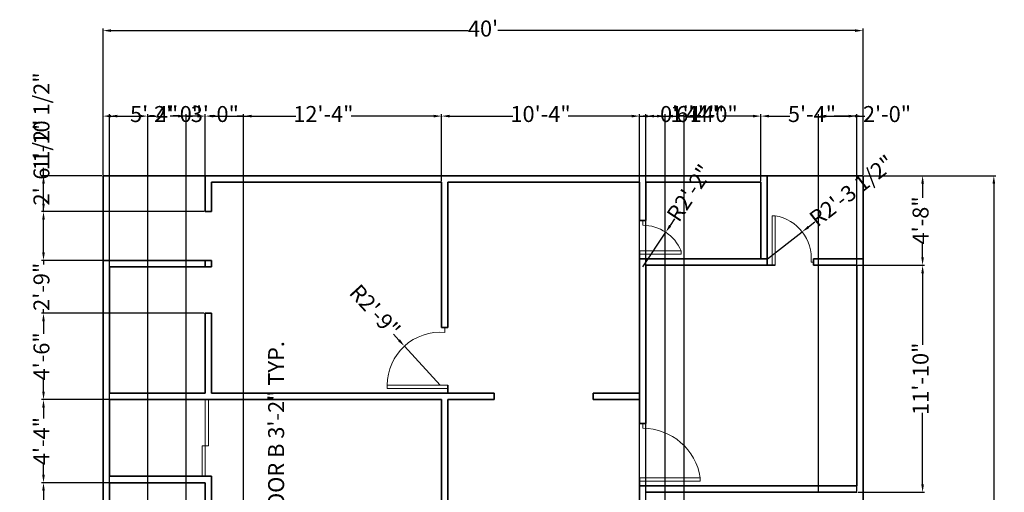
# Model space of a CAD drawing. Units: inches. Extents: x 2565 to 3182, y 2168 to 2957.
# Tile 3 of 3: x 2565 to 3182, y 2662 to 2957. Entities that reach past the tile are written whole.
import ezdxf

# ---------------------------------------------------------------- set-up
doc = ezdxf.new("R2010")
doc.units = ezdxf.units.IN
for name, color, linetype, lineweight in [('A-ANNO-DIMS', 2, 'Continuous', 13), ('A-DOOR', 4, 'Continuous', 18), ('A-GLAZ', 3, 'Continuous', 18), ('A-WALL', 7, 'Continuous', 35)]:
    doc.layers.add(name, color=color, linetype=linetype, lineweight=lineweight)
doc.styles.get("Standard").update_dxf_attribs({"font": 'arial.ttf'})
doc.dimstyles.new('ISO-25', dxfattribs={"dimtxt": 10, "dimasz": 5, "dimexe": 1.25, "dimexo": 0.625, "dimtad": 0, "dimdec": 0, "dimrnd": 10, "dimlunit": 3, "dimtxsty": 'Standard', "dimcen": 2.5, "dimadec": 0, "dimazin": 0, "dimtfac": 1, "dimtdec": 0, "dimtmove": 0, "dimatfit": 3, "dimfxl": 1, "dimarcsym": 0})

# ---------------------------------------------------------------- blocks, each defined once
blk = doc.blocks.new('*D2')
at = {"layer": 'A-ANNO-DIMS', "color": 0, "lineweight": -2, "transparency": 16777216}
for p, q in [((3094.05, 2859.77), (3176.57, 2859.77)), ((3175.32, 2854.77), (3175.32, 2553.57)), ((3175.32, 2216.77), (3175.32, 2517.97)), ((3094.05, 2211.77), (3176.57, 2211.77))]:
    blk.add_line(p, q, dxfattribs=at)
at = {"layer": 'A-ANNO-DIMS', "color": 0, "transparency": 16777216}
for points in [[(3174.49, 2854.77), (3176.15, 2854.77), (3175.32, 2859.77)], [(3174.49, 2216.77), (3176.15, 2216.77), (3175.32, 2211.77)]]:
    blk.add_solid(points, dxfattribs=at)
at = {"layer": 'Defpoints', "color": 0, "transparency": 16777216}
for p in [(3093.43, 2859.77), (3093.43, 2211.77), (3175.32, 2211.77)]:
    blk.add_point(p, dxfattribs=at)
at = {"layer": 'A-ANNO-DIMS', "color": 0, "transparency": 16777216, "insert": (3175.32, 2535.77), "char_height": 10, "attachment_point": 5, "rotation": 90}
blk.add_mtext('54\'-2"', dxfattribs=at)
blk = doc.blocks.new('*D3')
at = {"layer": 'A-ANNO-DIMS', "color": 0, "lineweight": -2, "transparency": 16777216}
for p, q in [((2617.43, 2860.39), (2617.43, 2951.77)), ((2622.43, 2950.52), (2846.12, 2950.52)), ((3088.43, 2950.52), (2864.74, 2950.52)), ((3093.43, 2860.39), (3093.43, 2951.77))]:
    blk.add_line(p, q, dxfattribs=at)
at = {"layer": 'A-ANNO-DIMS', "color": 0, "transparency": 16777216}
for points in [[(2622.43, 2951.35), (2622.43, 2949.69), (2617.43, 2950.52)], [(3088.43, 2951.35), (3088.43, 2949.69), (3093.43, 2950.52)]]:
    blk.add_solid(points, dxfattribs=at)
at = {"layer": 'Defpoints', "color": 0, "transparency": 16777216}
for p in [(3093.43, 2950.52), (2617.43, 2859.77), (3093.43, 2859.77)]:
    blk.add_point(p, dxfattribs=at)
at = {"layer": 'A-ANNO-DIMS', "color": 0, "transparency": 16777216, "insert": (2855.43, 2950.52), "char_height": 10, "attachment_point": 5}
blk.add_mtext("40'", dxfattribs=at)
blk = doc.blocks.new('DOOR-SWING-36-OPENING-39')
for p, q in [((2, 36), (2, 33)), ((38, 2), (0, 2)), ((0, 2), (0, 0)), ((2, 0), (38, 0)), ((38, 0), (38, 2))]:
    blk.add_line(p, q)
blk.add_arc((2, -3.4), 36.4, 8.53579, 90)
blk = doc.blocks.new('*D9')
at = {"layer": 'A-ANNO-DIMS', "color": 0, "lineweight": -2, "transparency": 16777216}
for p, q in [((2722.05, 2633.77), (2728.38, 2633.77)), ((2727.13, 2633.77), (2727.13, 2638.77)), ((2727.13, 2600.77), (2727.13, 2628.77)), ((2722.05, 2595.77), (2728.38, 2595.77))]:
    blk.add_line(p, q, dxfattribs=at)
at = {"layer": 'A-ANNO-DIMS', "color": 0, "transparency": 16777216}
for points in [[(2726.3, 2628.77), (2727.96, 2628.77), (2727.13, 2633.77)], [(2726.3, 2600.77), (2727.96, 2600.77), (2727.13, 2595.77)]]:
    blk.add_solid(points, dxfattribs=at)
at = {"layer": 'Defpoints', "color": 0, "transparency": 16777216}
for p in [(2721.43, 2633.77), (2727.13, 2633.77), (2721.43, 2595.77)]:
    blk.add_point(p, dxfattribs=at)
at = {"layer": 'A-ANNO-DIMS', "color": 0, "transparency": 16777216, "insert": (2727.13, 2699.12), "char_height": 10, "attachment_point": 5, "rotation": 90}
blk.add_mtext('DOOR B 3\'-2" TYP.', dxfattribs=at)
blk = doc.blocks.new('*D13')
at = {"layer": 'A-ANNO-DIMS', "color": 0, "lineweight": -2, "transparency": 16777216}
for p, q in [((2617.43, 2860.39), (2617.43, 2898.3)), ((2681.43, 2860.39), (2681.43, 2898.3)), ((2622.43, 2897.05), (2635.51, 2897.05)), ((2676.43, 2897.05), (2663.35, 2897.05))]:
    blk.add_line(p, q, dxfattribs=at)
at = {"layer": 'A-ANNO-DIMS', "color": 0, "transparency": 16777216}
for points in [[(2622.43, 2897.88), (2622.43, 2896.21), (2617.43, 2897.05)], [(2676.43, 2897.88), (2676.43, 2896.21), (2681.43, 2897.05)]]:
    blk.add_solid(points, dxfattribs=at)
at = {"layer": 'Defpoints', "color": 0, "transparency": 16777216}
for p in [(2681.43, 2897.05), (2617.43, 2859.77), (2681.43, 2859.77)]:
    blk.add_point(p, dxfattribs=at)
at = {"layer": 'A-ANNO-DIMS', "color": 0, "transparency": 16777216, "insert": (2649.43, 2897.05), "char_height": 10, "attachment_point": 5}
blk.add_mtext('5\'-4"', dxfattribs=at)
blk = doc.blocks.new('*D14')
at = {"layer": 'A-ANNO-DIMS', "color": 0, "lineweight": -2, "transparency": 16777216}
for p, q in [((2681.43, 2860.39), (2681.43, 2898.3)), ((2829.43, 2856.39), (2829.43, 2898.3)), ((2686.43, 2897.05), (2738.1, 2897.05)), ((2824.43, 2897.05), (2772.76, 2897.05))]:
    blk.add_line(p, q, dxfattribs=at)
at = {"layer": 'A-ANNO-DIMS', "color": 0, "transparency": 16777216}
for points in [[(2686.43, 2897.88), (2686.43, 2896.21), (2681.43, 2897.05)], [(2824.43, 2897.88), (2824.43, 2896.21), (2829.43, 2897.05)]]:
    blk.add_solid(points, dxfattribs=at)
at = {"layer": 'Defpoints', "color": 0, "transparency": 16777216}
for p in [(2829.43, 2897.05), (2681.43, 2859.77), (2829.43, 2855.77)]:
    blk.add_point(p, dxfattribs=at)
at = {"layer": 'A-ANNO-DIMS', "color": 0, "transparency": 16777216, "insert": (2755.43, 2897.05), "char_height": 10, "attachment_point": 5}
blk.add_mtext('12\'-4"', dxfattribs=at)
blk = doc.blocks.new('*D15')
at = {"layer": 'A-ANNO-DIMS', "color": 0, "lineweight": -2, "transparency": 16777216}
for p, q in [((2829.43, 2856.39), (2829.43, 2898.3)), ((2953.43, 2856.39), (2953.43, 2898.3)), ((2834.43, 2897.05), (2874.1, 2897.05)), ((2948.43, 2897.05), (2908.76, 2897.05))]:
    blk.add_line(p, q, dxfattribs=at)
at = {"layer": 'A-ANNO-DIMS', "color": 0, "transparency": 16777216}
for points in [[(2834.43, 2897.88), (2834.43, 2896.21), (2829.43, 2897.05)], [(2948.43, 2897.88), (2948.43, 2896.21), (2953.43, 2897.05)]]:
    blk.add_solid(points, dxfattribs=at)
at = {"layer": 'Defpoints', "color": 0, "transparency": 16777216}
for p in [(2953.43, 2897.05), (2829.43, 2855.77), (2953.43, 2855.77)]:
    blk.add_point(p, dxfattribs=at)
at = {"layer": 'A-ANNO-DIMS', "color": 0, "transparency": 16777216, "insert": (2891.43, 2897.05), "char_height": 10, "attachment_point": 5}
blk.add_mtext('10\'-4"', dxfattribs=at)
blk = doc.blocks.new('*D16')
at = {"layer": 'A-ANNO-DIMS', "color": 0, "lineweight": -2, "transparency": 16777216}
for p, q in [((2953.43, 2856.39), (2953.43, 2898.3)), ((3029.43, 2856.39), (3029.43, 2898.3)), ((2958.43, 2897.05), (2977.49, 2897.05)), ((3024.43, 2897.05), (3005.37, 2897.05))]:
    blk.add_line(p, q, dxfattribs=at)
at = {"layer": 'A-ANNO-DIMS', "color": 0, "transparency": 16777216}
for points in [[(2958.43, 2897.88), (2958.43, 2896.21), (2953.43, 2897.05)], [(3024.43, 2897.88), (3024.43, 2896.21), (3029.43, 2897.05)]]:
    blk.add_solid(points, dxfattribs=at)
at = {"layer": 'Defpoints', "color": 0, "transparency": 16777216}
for p in [(3029.43, 2897.05), (2953.43, 2855.77), (3029.43, 2855.77)]:
    blk.add_point(p, dxfattribs=at)
at = {"layer": 'A-ANNO-DIMS', "color": 0, "transparency": 16777216, "insert": (2991.43, 2897.05), "char_height": 10, "attachment_point": 5}
blk.add_mtext('6\'-4"', dxfattribs=at)
blk = doc.blocks.new('*D17')
at = {"layer": 'A-ANNO-DIMS', "color": 0, "lineweight": -2, "transparency": 16777216}
for p, q in [((3029.43, 2856.39), (3029.43, 2898.3)), ((3093.43, 2860.39), (3093.43, 2898.3)), ((3034.43, 2897.05), (3047.51, 2897.05)), ((3088.43, 2897.05), (3075.35, 2897.05))]:
    blk.add_line(p, q, dxfattribs=at)
at = {"layer": 'A-ANNO-DIMS', "color": 0, "transparency": 16777216}
for points in [[(3034.43, 2897.88), (3034.43, 2896.21), (3029.43, 2897.05)], [(3088.43, 2897.88), (3088.43, 2896.21), (3093.43, 2897.05)]]:
    blk.add_solid(points, dxfattribs=at)
at = {"layer": 'Defpoints', "color": 0, "transparency": 16777216}
for p in [(3093.43, 2897.05), (3029.43, 2855.77), (3093.43, 2859.77)]:
    blk.add_point(p, dxfattribs=at)
at = {"layer": 'A-ANNO-DIMS', "color": 0, "transparency": 16777216, "insert": (3061.43, 2897.05), "char_height": 10, "attachment_point": 5}
blk.add_mtext('5\'-4"', dxfattribs=at)
blk = doc.blocks.new('*D23')
at = {"layer": 'A-ANNO-DIMS', "color": 0, "lineweight": -2, "transparency": 16777216}
for p, q in [((2620.8, 2667.77), (2578.9, 2667.77)), ((2580.15, 2662.77), (2580.15, 2645.71)), ((2580.15, 2600.77), (2580.15, 2617.82)), ((2620.8, 2595.77), (2578.9, 2595.77))]:
    blk.add_line(p, q, dxfattribs=at)
at = {"layer": 'A-ANNO-DIMS', "color": 0, "transparency": 16777216}
for points in [[(2579.32, 2662.77), (2580.98, 2662.77), (2580.15, 2667.77)], [(2579.32, 2600.77), (2580.98, 2600.77), (2580.15, 2595.77)]]:
    blk.add_solid(points, dxfattribs=at)
at = {"layer": 'Defpoints', "color": 0, "transparency": 16777216}
for p in [(2580.15, 2667.77), (2621.43, 2667.77), (2621.43, 2595.77)]:
    blk.add_point(p, dxfattribs=at)
at = {"layer": 'A-ANNO-DIMS', "color": 0, "transparency": 16777216, "insert": (2580.15, 2631.77), "char_height": 10, "attachment_point": 5, "rotation": 90}
blk.add_mtext('6\'-0"', dxfattribs=at)
blk = doc.blocks.new('*D24')
at = {"layer": 'A-ANNO-DIMS', "color": 0, "lineweight": -2, "transparency": 16777216}
for p, q in [((2620.8, 2719.77), (2578.9, 2719.77)), ((2580.15, 2714.77), (2580.15, 2707.89)), ((2580.15, 2672.77), (2580.15, 2679.65)), ((2620.8, 2667.77), (2578.9, 2667.77))]:
    blk.add_line(p, q, dxfattribs=at)
at = {"layer": 'A-ANNO-DIMS', "color": 0, "transparency": 16777216}
for points in [[(2579.32, 2714.77), (2580.98, 2714.77), (2580.15, 2719.77)], [(2579.32, 2672.77), (2580.98, 2672.77), (2580.15, 2667.77)]]:
    blk.add_solid(points, dxfattribs=at)
at = {"layer": 'Defpoints', "color": 0, "transparency": 16777216}
for p in [(2580.15, 2719.77), (2621.43, 2719.77), (2621.43, 2667.77)]:
    blk.add_point(p, dxfattribs=at)
at = {"layer": 'A-ANNO-DIMS', "color": 0, "transparency": 16777216, "insert": (2580.15, 2693.77), "char_height": 10, "attachment_point": 5, "rotation": 90}
blk.add_mtext('4\'-4"', dxfattribs=at)
blk = doc.blocks.new('*D25')
at = {"layer": 'A-ANNO-DIMS', "color": 0, "lineweight": -2, "transparency": 16777216}
for p, q in [((2680.8, 2773.77), (2578.9, 2773.77)), ((2580.15, 2768.77), (2580.15, 2760.89)), ((2580.15, 2724.77), (2580.15, 2732.65)), ((2620.8, 2719.77), (2578.9, 2719.77))]:
    blk.add_line(p, q, dxfattribs=at)
at = {"layer": 'A-ANNO-DIMS', "color": 0, "transparency": 16777216}
for points in [[(2579.32, 2768.77), (2580.98, 2768.77), (2580.15, 2773.77)], [(2579.32, 2724.77), (2580.98, 2724.77), (2580.15, 2719.77)]]:
    blk.add_solid(points, dxfattribs=at)
at = {"layer": 'Defpoints', "color": 0, "transparency": 16777216}
for p in [(2580.15, 2773.77), (2681.43, 2773.77), (2621.43, 2719.77)]:
    blk.add_point(p, dxfattribs=at)
at = {"layer": 'A-ANNO-DIMS', "color": 0, "transparency": 16777216, "insert": (2580.15, 2746.77), "char_height": 10, "attachment_point": 5, "rotation": 90}
blk.add_mtext('4\'-6"', dxfattribs=at)
blk = doc.blocks.new('*D26')
at = {"layer": 'A-ANNO-DIMS', "color": 0, "lineweight": -2, "transparency": 16777216}
for p, q in [((2580.15, 2811.77), (2580.15, 2816.77)), ((2616.8, 2806.77), (2578.9, 2806.77)), ((2580.15, 2806.77), (2580.15, 2804.27)), ((2580.15, 2773.77), (2580.15, 2776.27)), ((2680.8, 2773.77), (2578.9, 2773.77)), ((2580.15, 2768.77), (2580.15, 2763.77))]:
    blk.add_line(p, q, dxfattribs=at)
at = {"layer": 'A-ANNO-DIMS', "color": 0, "transparency": 16777216}
for points in [[(2579.32, 2811.77), (2580.98, 2811.77), (2580.15, 2806.77)], [(2579.32, 2768.77), (2580.98, 2768.77), (2580.15, 2773.77)]]:
    blk.add_solid(points, dxfattribs=at)
at = {"layer": 'Defpoints', "color": 0, "transparency": 16777216}
for p in [(2580.15, 2806.77), (2617.43, 2806.77), (2681.43, 2773.77)]:
    blk.add_point(p, dxfattribs=at)
at = {"layer": 'A-ANNO-DIMS', "color": 0, "transparency": 16777216, "insert": (2580.15, 2790.27), "char_height": 10, "attachment_point": 5, "rotation": 90}
blk.add_mtext('2\'-9"', dxfattribs=at)
blk = doc.blocks.new('*D27')
at = {"layer": 'A-ANNO-DIMS', "color": 0, "lineweight": -2, "transparency": 16777216}
for p, q in [((2680.8, 2837.35), (2578.9, 2837.35)), ((2580.15, 2837.35), (2580.15, 2842.35)), ((2580.15, 2811.77), (2580.15, 2832.35)), ((2616.8, 2806.77), (2578.9, 2806.77))]:
    blk.add_line(p, q, dxfattribs=at)
at = {"layer": 'A-ANNO-DIMS', "color": 0, "transparency": 16777216}
for points in [[(2579.32, 2832.35), (2580.98, 2832.35), (2580.15, 2837.35)], [(2579.32, 2811.77), (2580.98, 2811.77), (2580.15, 2806.77)]]:
    blk.add_solid(points, dxfattribs=at)
at = {"layer": 'Defpoints', "color": 0, "transparency": 16777216}
for p in [(2580.15, 2837.35), (2681.43, 2837.35), (2617.43, 2806.77)]:
    blk.add_point(p, dxfattribs=at)
at = {"layer": 'A-ANNO-DIMS', "color": 0, "transparency": 16777216, "insert": (2580.15, 2868), "char_height": 10, "attachment_point": 5, "rotation": 90}
blk.add_mtext('2\'-6 1/2"', dxfattribs=at)
blk = doc.blocks.new('*D28')
at = {"layer": 'A-ANNO-DIMS', "color": 0, "lineweight": -2, "transparency": 16777216}
for p, q in [((2580.15, 2859.77), (2580.15, 2864.77)), ((2616.8, 2859.77), (2578.9, 2859.77)), ((2580.15, 2842.35), (2580.15, 2854.77)), ((2680.8, 2837.35), (2578.9, 2837.35))]:
    blk.add_line(p, q, dxfattribs=at)
at = {"layer": 'A-ANNO-DIMS', "color": 0, "transparency": 16777216}
for points in [[(2579.32, 2854.77), (2580.98, 2854.77), (2580.15, 2859.77)], [(2579.32, 2842.35), (2580.98, 2842.35), (2580.15, 2837.35)]]:
    blk.add_solid(points, dxfattribs=at)
at = {"layer": 'Defpoints', "color": 0, "transparency": 16777216}
for p in [(2580.15, 2859.77), (2617.43, 2859.77), (2681.43, 2837.35)]:
    blk.add_point(p, dxfattribs=at)
at = {"layer": 'A-ANNO-DIMS', "color": 0, "transparency": 16777216, "insert": (2580.15, 2893.75), "char_height": 10, "attachment_point": 5, "rotation": 90}
blk.add_mtext('1\'-10 1/2"', dxfattribs=at)
blk = doc.blocks.new('*D34')
at = {"layer": 'A-ANNO-DIMS', "color": 0, "lineweight": -2, "transparency": 16777216}
for p, q in [((3090.05, 2803.77), (3131.96, 2803.77)), ((3130.71, 2798.77), (3130.71, 2753.98)), ((3130.71, 2666.77), (3130.71, 2711.55)), ((3090.05, 2661.77), (3131.96, 2661.77))]:
    blk.add_line(p, q, dxfattribs=at)
at = {"layer": 'A-ANNO-DIMS', "color": 0, "transparency": 16777216}
for points in [[(3129.88, 2798.77), (3131.54, 2798.77), (3130.71, 2803.77)], [(3129.88, 2666.77), (3131.54, 2666.77), (3130.71, 2661.77)]]:
    blk.add_solid(points, dxfattribs=at)
at = {"layer": 'Defpoints', "color": 0, "transparency": 16777216}
for p in [(3089.43, 2803.77), (3130.71, 2803.77), (3089.43, 2661.77)]:
    blk.add_point(p, dxfattribs=at)
at = {"layer": 'A-ANNO-DIMS', "color": 0, "transparency": 16777216, "insert": (3130.71, 2732.77), "char_height": 10, "attachment_point": 5, "rotation": 90}
blk.add_mtext('11\'-10"', dxfattribs=at)
blk = doc.blocks.new('*D35')
at = {"layer": 'A-ANNO-DIMS', "color": 0, "lineweight": -2, "transparency": 16777216}
for p, q in [((3094.05, 2859.77), (3131.96, 2859.77)), ((3130.71, 2854.77), (3130.71, 2845.89)), ((3130.71, 2808.77), (3130.71, 2817.65)), ((3090.05, 2803.77), (3131.96, 2803.77))]:
    blk.add_line(p, q, dxfattribs=at)
at = {"layer": 'A-ANNO-DIMS', "color": 0, "transparency": 16777216}
for points in [[(3129.88, 2854.77), (3131.54, 2854.77), (3130.71, 2859.77)], [(3129.88, 2808.77), (3131.54, 2808.77), (3130.71, 2803.77)]]:
    blk.add_solid(points, dxfattribs=at)
at = {"layer": 'Defpoints', "color": 0, "transparency": 16777216}
for p in [(3093.43, 2859.77), (3130.71, 2859.77), (3089.43, 2803.77)]:
    blk.add_point(p, dxfattribs=at)
at = {"layer": 'A-ANNO-DIMS', "color": 0, "transparency": 16777216, "insert": (3130.71, 2831.77), "char_height": 10, "attachment_point": 5, "rotation": 90}
blk.add_mtext('4\'-8"', dxfattribs=at)
blk = doc.blocks.new('*D42')
at = {"layer": 'A-ANNO-DIMS', "color": 0, "lineweight": -2, "transparency": 16777216}
for p, q in [((2669.43, 2552.39), (2669.43, 2898.3)), ((2705.43, 2552.39), (2705.43, 2898.3)), ((2664.43, 2897.05), (2659.43, 2897.05)), ((2669.43, 2897.05), (2673.52, 2897.05)), ((2705.43, 2897.05), (2701.34, 2897.05)), ((2710.43, 2897.05), (2715.43, 2897.05))]:
    blk.add_line(p, q, dxfattribs=at)
at = {"layer": 'A-ANNO-DIMS', "color": 0, "transparency": 16777216}
for points in [[(2664.43, 2897.88), (2664.43, 2896.21), (2669.43, 2897.05)], [(2710.43, 2897.88), (2710.43, 2896.21), (2705.43, 2897.05)]]:
    blk.add_solid(points, dxfattribs=at)
at = {"layer": 'Defpoints', "color": 0, "transparency": 16777216}
for p in [(2705.43, 2897.05), (2669.43, 2551.77), (2705.43, 2551.77)]:
    blk.add_point(p, dxfattribs=at)
at = {"layer": 'A-ANNO-DIMS', "color": 0, "transparency": 16777216, "insert": (2687.43, 2897.05), "char_height": 10, "attachment_point": 5}
blk.add_mtext('3\'-0"', dxfattribs=at)
blk = doc.blocks.new('*D43')
at = {"layer": 'A-ANNO-DIMS', "color": 0, "lineweight": -2, "transparency": 16777216}
for p, q in [((2621.43, 2548.39), (2621.43, 2898.3)), ((2645.43, 2548.39), (2645.43, 2898.3)), ((2626.43, 2897.05), (2640.43, 2897.05)), ((2645.43, 2897.05), (2650.43, 2897.05))]:
    blk.add_line(p, q, dxfattribs=at)
at = {"layer": 'A-ANNO-DIMS', "color": 0, "transparency": 16777216}
for points in [[(2626.43, 2897.88), (2626.43, 2896.21), (2621.43, 2897.05)], [(2640.43, 2897.88), (2640.43, 2896.21), (2645.43, 2897.05)]]:
    blk.add_solid(points, dxfattribs=at)
at = {"layer": 'Defpoints', "color": 0, "transparency": 16777216}
for p in [(2645.43, 2897.05), (2621.43, 2547.77), (2645.43, 2547.77)]:
    blk.add_point(p, dxfattribs=at)
at = {"layer": 'A-ANNO-DIMS', "color": 0, "transparency": 16777216, "insert": (2664.43, 2897.05), "char_height": 10, "attachment_point": 5}
blk.add_mtext('2\'-0"', dxfattribs=at)
blk = doc.blocks.new('*D52')
at = {"layer": 'A-ANNO-DIMS', "color": 0, "lineweight": -2, "transparency": 16777216}
for p, q in [((2953.43, 2586.39), (2953.43, 2898.3)), ((2969.43, 2586.39), (2969.43, 2898.3)), ((2958.43, 2897.05), (2964.43, 2897.05)), ((2969.43, 2897.05), (2974.43, 2897.05))]:
    blk.add_line(p, q, dxfattribs=at)
at = {"layer": 'A-ANNO-DIMS', "color": 0, "transparency": 16777216}
for points in [[(2958.43, 2897.88), (2958.43, 2896.21), (2953.43, 2897.05)], [(2964.43, 2897.88), (2964.43, 2896.21), (2969.43, 2897.05)]]:
    blk.add_solid(points, dxfattribs=at)
at = {"layer": 'Defpoints', "color": 0, "transparency": 16777216}
for p in [(2969.43, 2897.05), (2953.43, 2585.77), (2969.43, 2585.77)]:
    blk.add_point(p, dxfattribs=at)
at = {"layer": 'A-ANNO-DIMS', "color": 0, "transparency": 16777216, "insert": (2987.87, 2897.05), "char_height": 10, "attachment_point": 5}
blk.add_mtext('1\'-4"', dxfattribs=at)
blk = doc.blocks.new('*D53')
at = {"layer": 'A-ANNO-DIMS', "color": 0, "lineweight": -2, "transparency": 16777216}
for p, q in [((2969.43, 2586.39), (2969.43, 2898.3)), ((2981.43, 2586.39), (2981.43, 2898.3)), ((2974.43, 2897.05), (2976.43, 2897.05)), ((2981.43, 2897.05), (2986.43, 2897.05))]:
    blk.add_line(p, q, dxfattribs=at)
at = {"layer": 'A-ANNO-DIMS', "color": 0, "transparency": 16777216}
for points in [[(2974.43, 2897.88), (2974.43, 2896.21), (2969.43, 2897.05)], [(2976.43, 2897.88), (2976.43, 2896.21), (2981.43, 2897.05)]]:
    blk.add_solid(points, dxfattribs=at)
at = {"layer": 'Defpoints', "color": 0, "transparency": 16777216}
for p in [(2981.43, 2897.05), (2969.43, 2585.77), (2981.43, 2585.77)]:
    blk.add_point(p, dxfattribs=at)
at = {"layer": 'A-ANNO-DIMS', "color": 0, "transparency": 16777216, "insert": (2999.87, 2897.05), "char_height": 10, "attachment_point": 5}
blk.add_mtext('1\'-0"', dxfattribs=at)
blk = doc.blocks.new('*D57')
at = {"layer": 'A-ANNO-DIMS', "color": 0, "lineweight": -2, "transparency": 16777216}
for p, q in [((3065.43, 2662.39), (3065.43, 2898.3)), ((3089.43, 2662.39), (3089.43, 2898.3)), ((3070.43, 2897.05), (3084.43, 2897.05)), ((3089.43, 2897.05), (3094.43, 2897.05))]:
    blk.add_line(p, q, dxfattribs=at)
at = {"layer": 'A-ANNO-DIMS', "color": 0, "transparency": 16777216}
for points in [[(3070.43, 2897.88), (3070.43, 2896.21), (3065.43, 2897.05)], [(3084.43, 2897.88), (3084.43, 2896.21), (3089.43, 2897.05)]]:
    blk.add_solid(points, dxfattribs=at)
at = {"layer": 'Defpoints', "color": 0, "transparency": 16777216}
for p in [(3089.43, 2897.05), (3065.43, 2661.77), (3089.43, 2661.77)]:
    blk.add_point(p, dxfattribs=at)
at = {"layer": 'A-ANNO-DIMS', "color": 0, "transparency": 16777216, "insert": (3108.43, 2897.05), "char_height": 10, "attachment_point": 5}
blk.add_mtext('2\'-0"', dxfattribs=at)
blk = doc.blocks.new('*D59')
at = {"layer": 'A-ANNO-DIMS', "color": 0, "lineweight": -2, "transparency": 16777216}
for p, q in [((2953.43, 2623.39), (2953.43, 2898.3)), ((2957.43, 2623.39), (2957.43, 2898.3)), ((2948.43, 2897.05), (2943.43, 2897.05)), ((2953.43, 2897.05), (2957.43, 2897.05)), ((2962.43, 2897.05), (2967.43, 2897.05))]:
    blk.add_line(p, q, dxfattribs=at)
at = {"layer": 'A-ANNO-DIMS', "color": 0, "transparency": 16777216}
for points in [[(2948.43, 2897.88), (2948.43, 2896.21), (2953.43, 2897.05)], [(2962.43, 2897.88), (2962.43, 2896.21), (2957.43, 2897.05)]]:
    blk.add_solid(points, dxfattribs=at)
at = {"layer": 'Defpoints', "color": 0, "transparency": 16777216}
for p in [(2957.43, 2897.05), (2953.43, 2622.77), (2957.43, 2622.77)]:
    blk.add_point(p, dxfattribs=at)
at = {"layer": 'A-ANNO-DIMS', "color": 0, "transparency": 16777216, "insert": (2981.35, 2897.05), "char_height": 10, "attachment_point": 5}
blk.add_mtext('0\'-4"', dxfattribs=at)
blk = doc.blocks.new('*D65')
at = {"layer": 'A-ANNO-DIMS', "color": 0, "lineweight": -2, "transparency": 16777216}
for p, q in [((2799.41, 2760.56), (2802.79, 2756.87)), ((2828.55, 2728.77), (2806.17, 2753.19))]:
    blk.add_line(p, q, dxfattribs=at)
at = {"layer": 'A-ANNO-DIMS', "color": 0, "transparency": 16777216}
blk.add_solid([(2803.41, 2757.44), (2802.18, 2756.31), (2806.17, 2753.19)], dxfattribs=at)
at = {"layer": 'Defpoints', "color": 0, "transparency": 16777216}
for p in [(2806.17, 2753.19), (2828.55, 2728.77)]:
    blk.add_point(p, dxfattribs=at)
at = {"layer": 'A-ANNO-DIMS', "color": 0, "transparency": 16777216, "insert": (2786.78, 2774.34), "char_height": 10, "attachment_point": 5, "rotation": 312.51029}
blk.add_mtext('R2\'-9"', dxfattribs=at)
blk = doc.blocks.new('*D69')
at = {"layer": 'A-ANNO-DIMS', "color": 0, "lineweight": -2, "transparency": 16777216}
for p, q in [((3063.17, 2830.74), (3059.22, 2827.67)), ((3033.67, 2807.85), (3055.27, 2824.61))]:
    blk.add_line(p, q, dxfattribs=at)
at = {"layer": 'A-ANNO-DIMS', "color": 0, "transparency": 16777216}
blk.add_solid([(3058.71, 2828.33), (3059.73, 2827.01), (3055.27, 2824.61)], dxfattribs=at)
at = {"layer": 'Defpoints', "color": 0, "transparency": 16777216}
for p in [(3055.27, 2824.61), (3033.67, 2807.85)]:
    blk.add_point(p, dxfattribs=at)
at = {"layer": 'A-ANNO-DIMS', "color": 0, "transparency": 16777216, "insert": (3087.15, 2849.34), "char_height": 10, "attachment_point": 5, "rotation": 37.80584}
blk.add_mtext('R2\'-3 1/2"', dxfattribs=at)
blk = doc.blocks.new('*D71')
at = {"layer": 'A-ANNO-DIMS', "color": 0, "lineweight": -2, "transparency": 16777216}
for p, q in [((2975.4, 2832.72), (2972.62, 2828.56)), ((2955.43, 2802.77), (2969.85, 2824.4))]:
    blk.add_line(p, q, dxfattribs=at)
at = {"layer": 'A-ANNO-DIMS', "color": 0, "transparency": 16777216}
blk.add_solid([(2971.93, 2829.02), (2973.32, 2828.1), (2969.85, 2824.4)], dxfattribs=at)
at = {"layer": 'Defpoints', "color": 0, "transparency": 16777216}
for p in [(2969.85, 2824.4), (2955.43, 2802.77)]:
    blk.add_point(p, dxfattribs=at)
at = {"layer": 'A-ANNO-DIMS', "color": 0, "transparency": 16777216, "insert": (2985.77, 2848.28), "char_height": 10, "attachment_point": 5, "rotation": 56.31031}
blk.add_mtext('R2\'-2"', dxfattribs=at)

msp = doc.modelspace()

# ---------------------------------------------------------------- linework, layer by layer
at = {"layer": 'A-DOOR'}
for p, q in [((2955.43, 2831.77), (2955.43, 2828.77)), ((3036.43, 2805.77), (3036.43, 2834.77)), ((3036.43, 2834.77), (3038.43, 2834.77)), ((3038.43, 2834.77), (3038.43, 2803.77)), ((2979.43, 2812.77), (2953.43, 2812.77)), ((2953.43, 2812.77), (2953.43, 2810.77)), ((2979.43, 2810.77), (2979.43, 2812.77)), ((2953.43, 2810.77), (2957.43, 2810.77)), ((2955.43, 2810.77), (2979.43, 2810.77)), ((3036.43, 2803.77), (3036.43, 2807.77)), ((3062.43, 2805.77), (3060.93, 2805.77)), ((3038.43, 2803.77), (3036.43, 2803.77)), ((2831.43, 2764.77), (2831.43, 2761.77)), ((2795.43, 2726.77), (2795.43, 2728.77)), ((2795.43, 2728.77), (2833.43, 2728.77)), ((2831.43, 2726.77), (2795.43, 2726.77)), ((2833.43, 2726.77), (2826.72, 2726.77)), ((2829.43, 2728.77), (2833.43, 2728.77)), ((2833.43, 2728.77), (2833.43, 2726.77)), ((2953.43, 2668.77), (2957.43, 2668.77))]:
    msp.add_line(p, q, dxfattribs=at)
for centre, radius, start, end in [((3033.67, 2807.85), 27.33, 355.631, 79.98206), ((2955.43, 2802.77), 26, 22.61986, 90), ((2828.55, 2728.77), 33.12, 85.02089, 180)]:
    msp.add_arc(centre, radius, start, end, dxfattribs=at)
at = {"layer": 'A-GLAZ'}
for p, q in [((2681.43, 2719.77), (2681.43, 2690.77)), ((2683.43, 2719.77), (2681.43, 2719.77)), ((2683.43, 2690.77), (2683.43, 2719.77)), ((2681.43, 2690.77), (2679.43, 2690.77)), ((2679.43, 2690.77), (2679.43, 2671.77)), ((2681.43, 2690.77), (2683.43, 2690.77)), ((2681.43, 2671.78), (2681.43, 2690.77)), ((2679.43, 2671.77), (2681.43, 2671.78))]:
    msp.add_line(p, q, dxfattribs=at)
at = {"layer": 'A-WALL'}
for p, q in [((3093.43, 2859.77), (2617.43, 2859.77)), ((2617.43, 2859.77), (2617.43, 2211.77)), ((2681.43, 2855.77), (2681.43, 2859.77)), ((2681.43, 2855.77), (2681.43, 2837.35)), ((2685.43, 2855.77), (2685.43, 2837.35)), ((2829.43, 2855.77), (2685.43, 2855.77)), ((2829.43, 2855.77), (2829.43, 2764.77)), ((2833.43, 2855.77), (2833.43, 2764.77)), ((2953.43, 2855.77), (2833.43, 2855.77)), ((2953.43, 2855.77), (2953.43, 2831.77)), ((3029.43, 2855.77), (2957.43, 2855.77)), ((2957.43, 2855.77), (2957.43, 2831.77)), ((3029.43, 2855.77), (3029.43, 2807.77)), ((3033.43, 2855.77), (3033.43, 2859.77)), ((3033.43, 2855.77), (3033.43, 2807.77)), ((3093.43, 2211.77), (3093.43, 2859.77)), ((2685.43, 2837.35), (2681.43, 2837.35)), ((2957.43, 2831.77), (2953.43, 2831.77)), ((2953.43, 2812.77), (2953.43, 2704.77)), ((2621.43, 2806.77), (2617.43, 2806.77)), ((2681.43, 2806.77), (2621.43, 2806.77)), ((2681.43, 2806.77), (2685.43, 2806.77)), ((2681.43, 2806.77), (2681.43, 2802.77)), ((2685.43, 2806.77), (2685.43, 2802.77)), ((2685.43, 2806.77), (2685.43, 2802.77)), ((2957.43, 2807.77), (2953.43, 2807.77)), ((3033.43, 2807.77), (2957.43, 2807.77)), ((3033.43, 2807.77), (3033.43, 2803.77)), ((3089.43, 2807.77), (3062.43, 2807.77)), ((3062.43, 2807.77), (3062.43, 2803.77)), ((3089.43, 2807.77), (3093.43, 2807.77)), ((2621.43, 2802.77), (2621.43, 2723.77)), ((2681.43, 2802.77), (2621.43, 2802.77)), ((2685.43, 2802.77), (2681.43, 2802.77)), ((2957.43, 2803.77), (2957.43, 2704.77)), ((3038.43, 2803.77), (2957.43, 2803.77)), ((3089.43, 2803.77), (3062.43, 2803.77)), ((3089.43, 2803.77), (3089.43, 2665.77)), ((3089.43, 2665.77), (3089.43, 2803.77)), ((2685.43, 2773.77), (2681.43, 2773.77)), ((2681.43, 2773.77), (2681.43, 2723.77)), ((2685.43, 2773.77), (2685.43, 2723.77)), ((2829.43, 2764.77), (2833.43, 2764.77)), ((2833.43, 2728.77), (2833.43, 2723.77)), ((2681.43, 2723.77), (2621.43, 2723.77)), ((2681.43, 2719.77), (2621.43, 2719.77)), ((2621.43, 2719.77), (2621.43, 2671.77)), ((2681.43, 2719.77), (2685.43, 2719.77)), ((2862.43, 2723.77), (2685.43, 2723.77)), ((2829.43, 2719.77), (2685.43, 2719.77)), ((2829.43, 2723.77), (2833.43, 2723.77)), ((2829.43, 2719.77), (2829.43, 2599.77)), ((2862.43, 2719.77), (2833.43, 2719.77)), ((2833.43, 2719.77), (2833.43, 2599.77)), ((2862.43, 2719.77), (2862.43, 2723.77)), ((2953.43, 2723.77), (2924.43, 2723.77)), ((2924.43, 2719.77), (2924.43, 2723.77)), ((2953.43, 2719.77), (2924.43, 2719.77)), ((2957.43, 2704.77), (2953.43, 2704.77)), ((2681.43, 2671.77), (2621.43, 2671.77)), ((2681.43, 2671.77), (2685.43, 2671.77)), ((2685.43, 2671.77), (2685.43, 2595.77)), ((2953.43, 2670.77), (2953.43, 2656.77)), ((2681.43, 2667.77), (2621.43, 2667.77)), ((2621.43, 2667.77), (2621.43, 2599.77)), ((2681.43, 2667.77), (2681.43, 2599.77)), ((2957.43, 2665.77), (2953.43, 2665.77)), ((3089.43, 2665.77), (2957.43, 2665.77)), ((3089.43, 2661.77), (2957.43, 2661.77))]:
    msp.add_line(p, q, dxfattribs=at)

# ---------------------------------------------------------------- block references
at = {"layer": 'A-DOOR'}
msp.add_blockref('DOOR-SWING-36-OPENING-39', (2953.43, 2668.77), dxfattribs=at)

# ---------------------------------------------------------------- dimensions: what is measured, and where the dimension line sits
at = {"layer": 'A-ANNO-DIMS'}
for base, p1, p2, override, picture, middle in [((3093.43, 2950.52), (2617.43, 2859.77), (3093.43, 2859.77), {"dimclrd": 0, "dimclre": 0, "dimclrt": 0}, '*D3', (2855.43, 2950.52)), ((2681.43, 2897.05), (2617.43, 2859.77), (2681.43, 2859.77), {"dimdec": 1, "dimlfac": 1, "dimrnd": 0, "dimzin": 1, "dimdsep": 46, "dimlunit": 4, "dimfrac": 2}, '*D13', (2649.43, 2897.05)), ((2645.43, 2897.05), (2621.43, 2547.77), (2645.43, 2547.77), {"dimdec": 1, "dimlfac": 1, "dimrnd": 0, "dimzin": 1, "dimdsep": 46, "dimlunit": 4, "dimfrac": 2}, '*D43', (2664.43, 2897.05)), ((2705.43, 2897.05), (2669.43, 2551.77), (2705.43, 2551.77), {"dimdec": 1, "dimlfac": 1, "dimrnd": 0, "dimzin": 1, "dimdsep": 46, "dimlunit": 4, "dimfrac": 2}, '*D42', (2687.43, 2897.05)), ((2829.43, 2897.05), (2681.43, 2859.77), (2829.43, 2855.77), {"dimdec": 1, "dimlfac": 1, "dimrnd": 0, "dimzin": 1, "dimdsep": 46, "dimlunit": 4, "dimfrac": 2}, '*D14', (2755.43, 2897.05)), ((2953.43, 2897.05), (2829.43, 2855.77), (2953.43, 2855.77), {"dimdec": 1, "dimlfac": 1, "dimrnd": 0, "dimzin": 1, "dimdsep": 46, "dimlunit": 4, "dimfrac": 2}, '*D15', (2891.43, 2897.05)), ((2957.43, 2897.05), (2953.43, 2622.77), (2957.43, 2622.77), {"dimdec": 1, "dimlfac": 1, "dimrnd": 0, "dimzin": 1, "dimdsep": 46, "dimlunit": 4, "dimfrac": 2}, '*D59', (2981.35, 2897.05)), ((3029.43, 2897.05), (2953.43, 2855.77), (3029.43, 2855.77), {"dimdec": 1, "dimlfac": 1, "dimrnd": 0, "dimzin": 1, "dimdsep": 46, "dimlunit": 4, "dimfrac": 2}, '*D16', (2991.43, 2897.05)), ((2969.43, 2897.05), (2953.43, 2585.77), (2969.43, 2585.77), {"dimdec": 1, "dimlfac": 1, "dimrnd": 0, "dimzin": 1, "dimdsep": 46, "dimlunit": 4, "dimfrac": 2}, '*D52', (2987.87, 2897.05)), ((2981.43, 2897.05), (2969.43, 2585.77), (2981.43, 2585.77), {"dimdec": 1, "dimlfac": 1, "dimrnd": 0, "dimzin": 1, "dimdsep": 46, "dimlunit": 4, "dimfrac": 2}, '*D53', (2999.87, 2897.05)), ((3093.43, 2897.05), (3029.43, 2855.77), (3093.43, 2859.77), {"dimdec": 1, "dimlfac": 1, "dimrnd": 0, "dimzin": 1, "dimdsep": 46, "dimlunit": 4, "dimfrac": 2}, '*D17', (3061.43, 2897.05)), ((3089.43, 2897.05), (3065.43, 2661.77), (3089.43, 2661.77), {"dimdec": 1, "dimlfac": 1, "dimrnd": 0, "dimzin": 1, "dimdsep": 46, "dimlunit": 4, "dimfrac": 2}, '*D57', (3108.43, 2897.05))]:
    dim = msp.add_linear_dim(base=base, p1=p1, p2=p2, dimstyle='ISO-25', override=override, dxfattribs=at)
    dim.commit()
    dim.dimension.update_dxf_attribs({"geometry": picture, "text_midpoint": middle})
for base, p1, p2, override, picture, middle in [((2580.15, 2859.77), (2681.43, 2837.35), (2617.43, 2859.77), {"dimdec": 1, "dimlfac": 1, "dimrnd": 0, "dimzin": 1, "dimdsep": 46, "dimlunit": 4, "dimfrac": 2}, '*D28', (2580.15, 2893.75)), ((2580.15, 2837.35), (2617.43, 2806.77), (2681.43, 2837.35), {"dimdec": 1, "dimlfac": 1, "dimrnd": 0, "dimzin": 1, "dimdsep": 46, "dimlunit": 4, "dimfrac": 2}, '*D27', (2580.15, 2868)), ((3130.71, 2859.77), (3089.43, 2803.77), (3093.43, 2859.77), {"dimdec": 1, "dimlfac": 1, "dimrnd": 0, "dimzin": 1, "dimdsep": 46, "dimlunit": 4, "dimfrac": 2}, '*D35', (3130.71, 2831.77)), ((3175.32, 2211.77), (3093.43, 2859.77), (3093.43, 2211.77), {"dimclrd": 0, "dimclre": 0, "dimclrt": 0}, '*D2', (3175.32, 2535.77)), ((2580.15, 2806.77), (2681.43, 2773.77), (2617.43, 2806.77), {"dimdec": 1, "dimlfac": 1, "dimrnd": 0, "dimzin": 1, "dimdsep": 46, "dimlunit": 4, "dimfrac": 2}, '*D26', (2580.15, 2790.27)), ((3130.71, 2803.77), (3089.43, 2661.77), (3089.43, 2803.77), {"dimdec": 1, "dimlfac": 1, "dimrnd": 0, "dimzin": 1, "dimdsep": 46, "dimlunit": 4, "dimfrac": 2}, '*D34', (3130.71, 2732.77)), ((2580.15, 2773.77), (2621.43, 2719.77), (2681.43, 2773.77), {"dimdec": 1, "dimlfac": 1, "dimrnd": 0, "dimzin": 1, "dimdsep": 46, "dimlunit": 4, "dimfrac": 2}, '*D25', (2580.15, 2746.77)), ((2580.15, 2719.77), (2621.43, 2667.77), (2621.43, 2719.77), {"dimdec": 1, "dimlfac": 1, "dimrnd": 0, "dimzin": 1, "dimdsep": 46, "dimlunit": 4, "dimfrac": 2}, '*D24', (2580.15, 2693.77)), ((2580.15, 2667.77), (2621.43, 2595.77), (2621.43, 2667.77), {"dimdec": 1, "dimlfac": 1, "dimrnd": 0, "dimzin": 1, "dimdsep": 46, "dimlunit": 4, "dimfrac": 2}, '*D23', (2580.15, 2631.77))]:
    dim = msp.add_linear_dim(base=base, p1=p1, p2=p2, angle=90, dimstyle='ISO-25', override=override, dxfattribs=at)
    dim.commit()
    dim.dimension.update_dxf_attribs({"geometry": picture, "text_midpoint": middle})
for center, mpoint, picture, middle in [((2955.43, 2802.77), (2969.85, 2824.4), '*D71', (2985.77, 2848.28)), ((3033.67, 2807.85), (3055.27, 2824.61), '*D69', (3087.15, 2849.34)), ((2828.55, 2728.77), (2806.17, 2753.19), '*D65', (2786.78, 2774.34))]:
    dim = msp.add_radius_dim(center=center, mpoint=mpoint, dimstyle='ISO-25', override={"dimdec": 1, "dimlfac": 1, "dimrnd": 0, "dimzin": 1, "dimdsep": 46, "dimlunit": 4, "dimfrac": 2}, dxfattribs=at)
    dim.commit()
    dim.dimension.update_dxf_attribs({"geometry": picture, "text_midpoint": middle})
dim = msp.add_linear_dim(base=(2727.13, 2633.77), p1=(2721.43, 2595.77), p2=(2721.43, 2633.77), angle=90, text='DOOR B <> TYP.', dimstyle='ISO-25', override={"dimdec": 1, "dimlfac": 1, "dimrnd": 0, "dimzin": 1, "dimdsep": 46, "dimlunit": 4, "dimfrac": 2}, dxfattribs=at)
dim.commit()
dim.dimension.update_dxf_attribs({"geometry": '*D9', "text_midpoint": (2727.13, 2699.12)})

doc.saveas('drawing.dxf')
